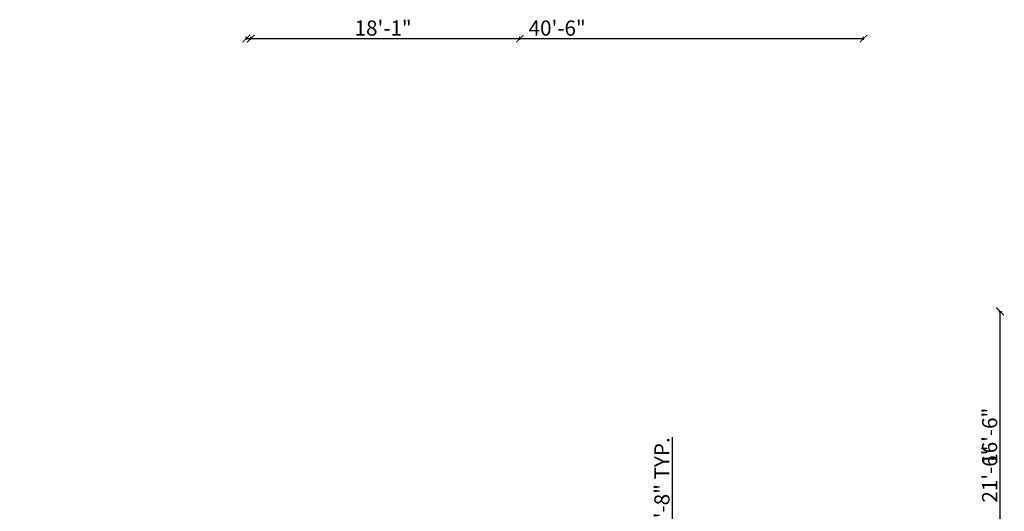
# Model space of a CAD drawing. Units: inches. Extents: x 261 to 2725, y 291 to 1454.
# Tile 35 of 35: x 1824 to 2605, y 1064 to 1454. Entities that reach past the tile are written whole.
import ezdxf

# ---------------------------------------------------------------- set-up
doc = ezdxf.new("R2010")
doc.units = ezdxf.units.IN
doc.layers.add('A-ANNO-DIMS', color=136, linetype='Continuous', lineweight=18)
doc.styles.get("Standard").update_dxf_attribs({"font": 'arial.ttf'})
doc.dimstyles.new('ISO-25', dxfattribs={"dimtxt": 12, "dimasz": 6, "dimexe": 1.25, "dimexo": 0.625, "dimtad": 1, "dimdec": 0, "dimlunit": 3, "dimtxsty": 'Standard', "dimblk": 'ARCHTICK', "dimcen": 2.5, "dimadec": 0, "dimazin": 0, "dimtfac": 1, "dimtdec": 0, "dimtmove": 0, "dimatfit": 3, "dimfxl": 1, "dimfxlon": 1, "dimarcsym": 0})

# ---------------------------------------------------------------- blocks, each defined once
blk = doc.blocks.new('_ArchTick')
at = {"color": 0, "linetype": 'ByBlock', "const_width": 0.15}
blk.add_lwpolyline([(-0.5, -0.5), (0.5, 0.5)], dxfattribs=at)
blk = doc.blocks.new('*D52')
at = {"layer": 'A-ANNO-DIMS', "color": 0, "lineweight": -2, "ltscale": 0.07, "transparency": 16777216}
for p, q in [((2342.06, 1043.35), (2342.06, 1122.62)), ((2343.06, 1043.35), (2340.81, 1043.35)), ((2342.06, 1023.35), (2342.06, 1043.35)), ((2343.06, 1023.35), (2340.81, 1023.35))]:
    blk.add_line(p, q, dxfattribs=at)
at = {"layer": 'Defpoints', "color": 0, "ltscale": 0.07, "transparency": 16777216}
for p in [(2342.06, 1043.35), (2348.5, 1043.35), (2348.5, 1023.35)]:
    blk.add_point(p, dxfattribs=at)
at = {"layer": 'A-ANNO-DIMS', "color": 0, "lineweight": -2, "ltscale": 0.07, "transparency": 16777216, "xscale": 6, "yscale": 6, "zscale": 6}
for p, rotation in [((2342.06, 1043.35), 90), ((2342.06, 1023.35), 270)]:
    blk.add_blockref('_ArchTick', p, dxfattribs=dict(at, rotation=rotation))
at = {"layer": 'A-ANNO-DIMS', "color": 0, "ltscale": 0.07, "transparency": 16777216, "insert": (2335.31, 1085.99), "char_height": 12, "attachment_point": 5, "rotation": 90}
blk.add_mtext('1\'-8" TYP.', dxfattribs=at)
blk = doc.blocks.new('*D85')
at = {"layer": 'A-ANNO-DIMS', "color": 0, "lineweight": -2, "ltscale": 0.07, "transparency": 16777216}
for p, q in [((2600.96, 1222.47), (2603.21, 1222.47)), ((2601.96, 1024.47), (2601.96, 1222.47)), ((2600.96, 1024.47), (2603.21, 1024.47))]:
    blk.add_line(p, q, dxfattribs=at)
at = {"layer": 'Defpoints', "color": 0, "ltscale": 0.07, "transparency": 16777216}
for p in [(946.45, 1222.47), (2601.96, 1222.47), (946.45, 1024.47)]:
    blk.add_point(p, dxfattribs=at)
at = {"layer": 'A-ANNO-DIMS', "color": 0, "lineweight": -2, "ltscale": 0.07, "transparency": 16777216, "xscale": 6, "yscale": 6, "zscale": 6}
for p, rotation in [((2601.96, 1222.47), 90), ((2601.96, 1024.47), 270)]:
    blk.add_blockref('_ArchTick', p, dxfattribs=dict(at, rotation=rotation))
at = {"layer": 'A-ANNO-DIMS', "color": 0, "ltscale": 0.07, "transparency": 16777216, "insert": (2595.21, 1123.47), "char_height": 12, "attachment_point": 5, "rotation": 90}
blk.add_mtext('16\'-6"', dxfattribs=at)
blk = doc.blocks.new('*D115')
at = {"layer": 'A-ANNO-DIMS', "color": 0, "lineweight": -2, "ltscale": 0.07, "transparency": 16777216}
for p, q in [((2600.96, 1222.47), (2603.21, 1222.47)), ((2601.96, 964.47), (2601.96, 1222.47)), ((2600.96, 964.47), (2603.21, 964.47))]:
    blk.add_line(p, q, dxfattribs=at)
at = {"layer": 'Defpoints', "color": 0, "ltscale": 0.07, "transparency": 16777216}
for p in [(1720.08, 1222.47), (2601.96, 1222.47), (1720.08, 964.47)]:
    blk.add_point(p, dxfattribs=at)
at = {"layer": 'A-ANNO-DIMS', "color": 0, "lineweight": -2, "ltscale": 0.07, "transparency": 16777216, "xscale": 6, "yscale": 6, "zscale": 6}
for p, rotation in [((2601.96, 1222.47), 90), ((2601.96, 964.47), 270)]:
    blk.add_blockref('_ArchTick', p, dxfattribs=dict(at, rotation=rotation))
at = {"layer": 'A-ANNO-DIMS', "color": 0, "ltscale": 0.07, "transparency": 16777216, "insert": (2595.21, 1093.47), "char_height": 12, "attachment_point": 5, "rotation": 90}
blk.add_mtext('21\'-6"', dxfattribs=at)
blk = doc.blocks.new('*D122')
at = {"layer": 'A-ANNO-DIMS', "color": 0, "lineweight": -2, "ltscale": 0.07, "transparency": 16777216}
for p, q in [((2007.71, 1437.76), (2007.71, 1440.01)), ((2007.71, 1438.76), (2493.71, 1438.76)), ((2493.71, 1437.76), (2493.71, 1440.01))]:
    blk.add_line(p, q, dxfattribs=at)
at = {"layer": 'Defpoints', "color": 0, "ltscale": 0.07, "transparency": 16777216}
for p in [(2493.71, 1438.76), (2007.71, 1054.85), (2493.71, 1054.85)]:
    blk.add_point(p, dxfattribs=at)
at = {"layer": 'A-ANNO-DIMS', "color": 0, "lineweight": -2, "ltscale": 0.07, "transparency": 16777216, "xscale": 6, "yscale": 6, "zscale": 6, "rotation": 180}
blk.add_blockref('_ArchTick', (2007.71, 1438.76), dxfattribs=at)
at = {"layer": 'A-ANNO-DIMS', "color": 0, "lineweight": -2, "ltscale": 0.07, "transparency": 16777216, "xscale": 6, "yscale": 6, "zscale": 6}
blk.add_blockref('_ArchTick', (2493.71, 1438.76), dxfattribs=at)
at = {"layer": 'A-ANNO-DIMS', "color": 0, "ltscale": 0.07, "transparency": 16777216, "insert": (2250.71, 1445.51), "char_height": 12, "attachment_point": 5}
blk.add_mtext('40\'-6"', dxfattribs=at)
blk = doc.blocks.new('*D135')
at = {"layer": 'A-ANNO-DIMS', "color": 0, "lineweight": -2, "ltscale": 0.07, "transparency": 16777216}
for p, q in [((2004.19, 1437.76), (2004.19, 1440.01)), ((2004.19, 1438.76), (2221.19, 1438.76)), ((2221.19, 1437.76), (2221.19, 1440.01))]:
    blk.add_line(p, q, dxfattribs=at)
at = {"layer": 'Defpoints', "color": 0, "ltscale": 0.07, "transparency": 16777216}
for p in [(2221.19, 1438.76), (2004.19, 642.39), (2221.19, 642.39)]:
    blk.add_point(p, dxfattribs=at)
at = {"layer": 'A-ANNO-DIMS', "color": 0, "lineweight": -2, "ltscale": 0.07, "transparency": 16777216, "xscale": 6, "yscale": 6, "zscale": 6, "rotation": 180}
blk.add_blockref('_ArchTick', (2004.19, 1438.76), dxfattribs=at)
at = {"layer": 'A-ANNO-DIMS', "color": 0, "lineweight": -2, "ltscale": 0.07, "transparency": 16777216, "xscale": 6, "yscale": 6, "zscale": 6}
blk.add_blockref('_ArchTick', (2221.19, 1438.76), dxfattribs=at)
at = {"layer": 'A-ANNO-DIMS', "color": 0, "ltscale": 0.07, "transparency": 16777216, "insert": (2112.69, 1445.51), "char_height": 12, "attachment_point": 5}
blk.add_mtext('18\'-1"', dxfattribs=at)

msp = doc.modelspace()

# ---------------------------------------------------------------- dimensions: what is measured, and where the dimension line sits
at = {"layer": 'A-ANNO-DIMS', "ltscale": 0.07}
for base, p1, p2, picture, middle in [((2221.19, 1438.76), (2004.19, 642.39), (2221.19, 642.39), '*D135', (2112.69, 1445.51)), ((2493.71, 1438.76), (2007.71, 1054.85), (2493.71, 1054.85), '*D122', (2250.71, 1445.51))]:
    dim = msp.add_linear_dim(base=base, p1=p1, p2=p2, dimstyle='ISO-25', override={"dimdec": 1, "dimlfac": 1, "dimrnd": 0, "dimzin": 1, "dimdsep": 46, "dimlunit": 4, "dimfrac": 2}, dxfattribs=at)
    dim.commit()
    dim.dimension.update_dxf_attribs({"geometry": picture, "text_midpoint": middle})
for p1, p2, picture, middle in [((946.45, 1024.47), (946.45, 1222.47), '*D85', (2595.21, 1123.47)), ((1720.08, 964.47), (1720.08, 1222.47), '*D115', (2595.21, 1093.47))]:
    dim = msp.add_linear_dim(base=(2601.96, 1222.47), p1=p1, p2=p2, angle=90, dimstyle='ISO-25', override={"dimdec": 1, "dimlfac": 1, "dimrnd": 0, "dimzin": 1, "dimdsep": 46, "dimlunit": 4, "dimfrac": 2}, dxfattribs=at)
    dim.commit()
    dim.dimension.update_dxf_attribs({"geometry": picture, "text_midpoint": middle})
dim = msp.add_linear_dim(base=(2342.06, 1043.35), p1=(2348.5, 1023.35), p2=(2348.5, 1043.35), angle=90, text='<> TYP.', dimstyle='ISO-25', override={"dimdec": 1, "dimrnd": 0, "dimzin": 1, "dimlunit": 4, "dimfrac": 2}, dxfattribs=at)
dim.commit()
dim.dimension.update_dxf_attribs({"geometry": '*D52', "text_midpoint": (2335.31, 1085.99)})

doc.saveas('drawing.dxf')
